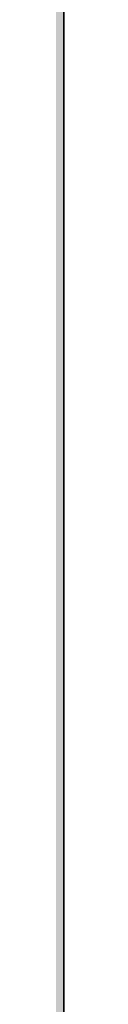
# Model space of a CAD drawing. Units: inches. Extents: x 2083 to 3317, y 1141 to 2115.
# Tile 205 of 256: x 3126.9598 to 3126.9598, y 1263.6134 to 1264.1307. Entities that reach past the tile are written whole.
import ezdxf

# ---------------------------------------------------------------- set-up
doc = ezdxf.new("R2010")
doc.units = ezdxf.units.IN
doc.layers.add('A-ANNO-DIMS', color=2, linetype='Continuous', lineweight=18)
doc.layers.add('A-WALL', color=7, linetype='Continuous', lineweight=35)
doc.layers.add('A-WALL-PATT', color=251, linetype='Continuous', lineweight=13, true_color=0x636466)
doc.styles.get("Standard").update_dxf_attribs({"font": 'arial.ttf'})
doc.dimstyles.new('ISO-25', dxfattribs={"dimtxt": 12, "dimasz": 12, "dimexe": 1.25, "dimexo": 0.625, "dimtad": 1, "dimlunit": 3, "dimtxsty": 'Standard', "dimcen": 2.5, "dimadec": 0, "dimazin": 0, "dimtfac": 1, "dimtmove": 0, "dimatfit": 3, "dimfxl": 1, "dimarcsym": 0})

# ---------------------------------------------------------------- blocks, each defined once
blk = doc.blocks.new('*D9')
at = {"layer": 'A-ANNO-DIMS', "color": 0, "lineweight": -2, "transparency": 16777216}
for p, q in [((3127.58478, 1486.76136), (3190.40309, 1486.76136)), ((3189.15309, 1474.76136), (3189.15309, 1275.26136)), ((3127.58478, 1263.26136), (3190.40309, 1263.26136))]:
    blk.add_line(p, q, dxfattribs=at)
at = {"layer": 'A-ANNO-DIMS', "color": 0, "transparency": 16777216}
for points in [[(3187.15309, 1474.76136), (3191.15309, 1474.76136), (3189.15309, 1486.76136)], [(3187.15309, 1275.26136), (3191.15309, 1275.26136), (3189.15309, 1263.26136)]]:
    blk.add_solid(points, dxfattribs=at)
at = {"layer": 'Defpoints', "color": 0, "transparency": 16777216}
for p in [(3126.95978, 1486.76136), (3126.95978, 1263.26136), (3189.15309, 1263.26136)]:
    blk.add_point(p, dxfattribs=at)
at = {"layer": 'A-ANNO-DIMS', "color": 0, "transparency": 16777216, "insert": (3182.40121, 1375.01136), "char_height": 12, "attachment_point": 5, "rotation": 90}
blk.add_mtext('18\'-7.5"', dxfattribs=at)
blk = doc.blocks.new('*D26')
at = {"layer": 'A-ANNO-DIMS', "color": 0, "lineweight": -2, "transparency": 16777216}
for p, q in [((3088.98584, 1274.91509), (3088.98584, 1270.95196)), ((3111.24004, 1274.91509), (3111.24004, 1270.95196)), ((3076.98584, 1272.20196), (2840.26245, 1272.20196)), ((3111.24004, 1272.20196), (3088.98584, 1272.20196)), ((3123.24004, 1272.20196), (3135.24004, 1272.20196))]:
    blk.add_line(p, q, dxfattribs=at)
at = {"layer": 'A-ANNO-DIMS', "color": 0, "transparency": 16777216}
for points in [[(3076.98584, 1274.20196), (3076.98584, 1270.20196), (3088.98584, 1272.20196)], [(3123.24004, 1274.20196), (3123.24004, 1270.20196), (3111.24004, 1272.20196)]]:
    blk.add_solid(points, dxfattribs=at)
at = {"layer": 'Defpoints', "color": 0, "transparency": 16777216}
for p in [(3088.98584, 1275.54009), (3111.24004, 1275.54009), (3088.98584, 1272.20196)]:
    blk.add_point(p, dxfattribs=at)
at = {"layer": 'A-ANNO-DIMS', "color": 0, "transparency": 16777216, "insert": (2952.62415, 1279.0316), "char_height": 12, "attachment_point": 5}
blk.add_mtext('NIGHTSTAND 1\'-10 1/2" TYP.', dxfattribs=at)
blk = doc.blocks.new('*D27')
at = {"layer": 'A-ANNO-DIMS', "color": 0, "lineweight": -2, "transparency": 16777216}
for p, q in [((3114.57817, 1309.79428), (3114.57817, 1321.79428)), ((3111.86504, 1297.79428), (3115.82817, 1297.79428)), ((3114.57817, 1297.79428), (3114.57817, 1275.54009)), ((3111.86504, 1275.54009), (3115.82817, 1275.54009)), ((3114.57817, 1263.54009), (3114.57817, 1140.98859))]:
    blk.add_line(p, q, dxfattribs=at)
at = {"layer": 'A-ANNO-DIMS', "color": 0, "transparency": 16777216}
for points in [[(3112.57817, 1309.79428), (3116.57817, 1309.79428), (3114.57817, 1297.79428)], [(3112.57817, 1263.54009), (3116.57817, 1263.54009), (3114.57817, 1275.54009)]]:
    blk.add_solid(points, dxfattribs=at)
at = {"layer": 'Defpoints', "color": 0, "transparency": 16777216}
for p in [(3111.24004, 1297.79428), (3111.24004, 1275.54009), (3114.57817, 1275.54009)]:
    blk.add_point(p, dxfattribs=at)
at = {"layer": 'A-ANNO-DIMS', "color": 0, "transparency": 16777216, "insert": (3107.74853, 1196.26434), "char_height": 12, "attachment_point": 5, "rotation": 90}
blk.add_mtext('1\'-10 1/2" TYP.', dxfattribs=at)

msp = doc.modelspace()

# ---------------------------------------------------------------- hatches: boundary and pattern name
at = {"layer": 'A-WALL-PATT'}
h = msp.add_hatch(color=256, dxfattribs=at)
h.dxf.hatch_style = 1
h.paths.add_polyline_path([(3126.95978, 2020.76136), (2748.95978, 2020.76136), (2604.95978, 2020.76136), (2226.95978, 2020.76136), (2226.95978, 1702.76136), (2466.95978, 1702.76136), (2466.95978, 1582.76136), (2418.95978, 1582.76136), (2418.95978, 1477.76136), (2226.95978, 1477.76136), (2226.95978, 1263.26136), (2544.95978, 1263.26136), (2544.95978, 1411.76136), (2604.95978, 1411.76136), (2685.95978, 1411.76136), (2685.95978, 1420.76136), (2604.95978, 1420.76136), (2604.95978, 1573.76136), (2604.95978, 1702.76136), (2604.95978, 2011.76136), (2748.95978, 2011.76136), (2748.95978, 1702.76136), (2862.95978, 1702.76136), (2862.95978, 1621.76136), (2871.95978, 1621.76136), (2871.95978, 1702.76136), (2883.95978, 1702.76136), (2883.95978, 1706.93946, -0.026459), (2883.95978, 1711.76136), (2757.95978, 1711.76136), (2757.95978, 1807.76136), (2787.95978, 1807.76136), (2787.95978, 1812.26136), (2757.95978, 1812.26136), (2757.95978, 2011.76136), (2877.95978, 2011.76136), (2877.95978, 1812.26136), (2847.95978, 1812.26136), (2847.95978, 1807.76136), (2889.83574, 1807.76136), (2889.83574, 1812.26136), (2882.45978, 1812.26136), (2882.45978, 2011.76136), (3117.95978, 2011.76136), (3117.95978, 1812.26136), (2937.83574, 1812.26136), (2937.83574, 1807.76136), (2995.70978, 1807.76136), (2995.70978, 1796.11767), (3000.20978, 1796.11767), (3000.20978, 1807.76136), (3117.95978, 1807.76136), (3117.95978, 1711.76136), (3000.20978, 1711.76136), (3000.20978, 1760.11767), (2998.5727, 1760.11767, -0.020711), (2995.70978, 1760.11767), (2995.70978, 1711.76136), (2931.95978, 1711.76136), (2931.95978, 1702.76136), (3126.95978, 1702.76136)])
h.paths.add_polyline_path([(2471.45978, 2011.76136), (2471.45978, 1810.01136), (2462.71694, 1810.01136), (2462.71694, 1805.51136), (2505.95978, 1805.51136), (2505.95978, 1810.01136), (2475.95978, 1810.01136), (2475.95978, 2011.76136), (2595.95978, 2011.76136), (2595.95978, 1810.01136), (2565.95978, 1810.01136), (2565.95978, 1805.51136), (2595.95978, 1805.51136), (2595.95978, 1711.76136), (2235.95978, 1711.76136), (2235.95978, 1805.51136), (2353.70978, 1805.51136), (2353.70978, 1796.05416), (2358.20978, 1796.05416), (2358.20978, 1805.51136), (2414.71694, 1805.51136), (2414.71694, 1810.01136), (2235.95978, 1810.01136), (2235.95978, 2011.76136)], flags=16)
h.paths.add_polyline_path([(2270.20473, 1994.61001), (2270.20473, 1970.61001), (2246.20473, 1970.61001), (2246.20473, 1994.61001)], flags=0)
edge = h.paths.add_edge_path(flags=0)
edge.add_ellipse((2332.02739, 1899.79818), major_axis=(-3.04299, 3.04299), ratio=0.1682525, start_angle=-161.33217, end_angle=-156.30711, ccw=False)
edge.add_ellipse((2333.08204, 1898.74353), major_axis=(-1.05465, 1.05465), ratio=0.4535321, start_angle=-123.37102, end_angle=-94.15911)
edge = h.paths.add_edge_path(flags=0)
edge.add_ellipse((2332.02739, 1968.87629), major_axis=(3.04299, 3.04299), ratio=0.1682525, start_angle=18.66783, end_angle=23.69289)
edge.add_spline(control_points=[(2332.9256, 1970.6911), (2332.22677, 1970.3361), (2330.89371, 1969.65891), (2328.41308, 1970.93214), (2327.20393, 1967.74871), (2324.7096, 1969.95559), (2322.53282, 1967.01235), (2320.01285, 1971.29581), (2317.68031, 1968.15784), (2316.04053, 1967.10205), (2315.4269, 1966.8096)], knot_values=[0, 0, 0, 0, 2.267059, 4.324559, 6.685584, 8.878641, 11.121502, 14.300359, 17.755284, 19.732645, 19.732645, 19.732645, 19.732645], degree=3, periodic=0)
edge.add_ellipse((2332.02739, 1968.87629), major_axis=(3.04299, 3.04299), ratio=0.1682525, start_angle=18.66783, end_angle=23.69289, ccw=False)
edge.add_ellipse((2333.08204, 1969.93094), major_axis=(1.05465, 1.05465), ratio=0.4535321, start_angle=56.62898, end_angle=85.84089, ccw=False)
edge = h.paths.add_edge_path(flags=0)
edge.add_spline(control_points=[(2296.42829, 1967.98791), (2293.6278, 1965.33631), (2287.70362, 1959.72709), (2299.74386, 1949.9957), (2294.53259, 1935.66853), (2290.57323, 1920.60351), (2293.39412, 1909.97369), (2296.18541, 1904.96654)], knot_values=[0.099185, 0.099185, 0.099185, 0.099185, 0.345301, 0.619822, 0.982653, 1.386093, 1.810555, 1.810555, 1.810555, 1.810555], degree=3, periodic=0)
edge.add_spline(control_points=[(2296.18541, 1904.96654), (2297.38358, 1902.6193), (2298.00097, 1901.94931), (2298.55297, 1901.46815)], knot_values=[0.006246, 0.006246, 0.006246, 0.006246, 0.055476, 0.055476, 0.055476, 0.055476], degree=3, periodic=0)
edge.add_spline(control_points=[(2298.55297, 1901.46815), (2297.25861, 1900.92322), (2295.22529, 1900.23213), (2293.06023, 1900.61421), (2292.10142, 1900.78841), (2292.08958, 1900.79057)], knot_values=[0.312835, 0.312835, 0.312835, 0.312835, 0.40178, 0.474987, 0.475903, 0.475903, 0.475903, 0.475903], degree=3, periodic=0)
edge.add_arc((2292.79365, 1904.66411), 3.93701, 215.4209, 259.69818, ccw=False)
edge.add_spline(control_points=[(2289.58531, 1902.3823), (2289.47665, 1902.53509), (2289.36848, 1902.68804), (2289.26086, 1902.84117)], knot_values=[0.102872, 0.102872, 0.102872, 0.102872, 0.116896, 0.116896, 0.116896, 0.116896], degree=3, periodic=0)
edge.add_spline(control_points=[(2289.26086, 1902.84117), (2288.6866, 1902.55019), (2287.64005, 1902.0199), (2285.88134, 1901.87395), (2283.85297, 1901.50435), (2281.71999, 1899.71054), (2278.46699, 1899.49294), (2276.15714, 1901.8832), (2272.25895, 1899.80407), (2267.77761, 1901.84318), (2262.24388, 1900.18403), (2257.41493, 1901.78206), (2254.31837, 1900.72612), (2253.17828, 1900.33734)], knot_values=[0, 0, 0, 0, 1.907977, 3.477176, 5.261074, 7.972851, 11.680248, 13.717921, 16.939592, 22.789562, 27.502503, 33.595215, 37.145618, 37.145618, 37.145618, 37.145618], degree=3, periodic=0)
edge.add_line((2253.17828, 1900.33734), (2250.24424, 1902.84117))
edge.add_line((2250.24424, 1902.84117), (2250.24424, 1965.8333))
edge.add_line((2250.24424, 1965.8333), (2253.17828, 1968.33712))
edge.add_spline(control_points=[(2253.17828, 1968.33712), (2254.31837, 1967.94835), (2257.41493, 1966.89241), (2262.24388, 1968.49043), (2267.77761, 1966.83128), (2271.52673, 1968.53722), (2273.87591, 1967.82829), (2274.2067, 1967.72764)], knot_values=[0, 0, 0, 0, 0.09018, 0.244935, 0.364644, 0.513233, 0.537855, 0.537855, 0.537855, 0.537855], degree=3, periodic=0)
edge.add_arc((2274.35289, 1963.79335), 3.93701, 72.05113, 92.12795, ccw=False)
edge.add_arc((2281.29693, 1985.23), 18.5963, 252.051134, 288.565722)
edge.add_arc((2292.31672, 1956.02888), 12.64608, 71.026788, 113.778218, ccw=False)
edge = h.paths.add_edge_path(flags=0)
edge.add_spline(control_points=[(2274.89941, 1951.85619), (2275.06616, 1951.61659), (2275.23269, 1951.37659), (2275.39799, 1951.13585)], knot_values=[1.409916, 1.409916, 1.409916, 1.409916, 1.43159, 1.43159, 1.43159, 1.43159], degree=3, periodic=0)
edge.add_spline(control_points=[(2275.39799, 1951.13585), (2275.79211, 1950.56189), (2276.17923, 1949.98377), (2276.54555, 1949.3971)], knot_values=[1.358238, 1.358238, 1.358238, 1.358238, 1.409916, 1.409916, 1.409916, 1.409916], degree=3, periodic=0)
edge.add_line((2276.54555, 1949.3971), (2277.43729, 1947.86218))
edge.add_spline(control_points=[(2277.43729, 1947.86218), (2276.30383, 1945.67311), (2274.6397, 1942.42688), (2274.63161, 1938.0939), (2272.79912, 1930.85155), (2274.35643, 1943.89705), (2275.94768, 1947.92336), (2276.54555, 1949.3971)], knot_values=[0.005632, 0.005632, 0.005632, 0.005632, 0.186014, 0.266002, 0.357087, 0.59639, 0.739732, 0.739732, 0.739732, 0.739732], degree=3, periodic=0)
edge.add_spline(control_points=[(2276.54555, 1949.3971), (2276.17923, 1949.98377), (2275.79211, 1950.56189), (2275.39799, 1951.13585)], knot_values=[1.358238, 1.358238, 1.358238, 1.358238, 1.409916, 1.409916, 1.409916, 1.409916], degree=3, periodic=0)
edge.add_spline(control_points=[(2275.39799, 1951.13585), (2274.9425, 1950.08045), (2274.20776, 1948.02527), (2273.9346, 1944.85148), (2272.46853, 1937.62749), (2273.46622, 1945.69647), (2274.70062, 1951.05947), (2274.89941, 1951.85619)], knot_values=[0.104364, 0.104364, 0.104364, 0.104364, 0.189636, 0.269624, 0.36071, 0.600013, 0.644622, 0.644622, 0.644622, 0.644622], degree=3, periodic=0)
h.paths.add_polyline_path([(2269.16751, 1963.12757, -0.357527), (2268.17063, 1960.97637, -0.092561), (2268.17063, 1939.43632, -0.357527), (2269.16751, 1937.28512, -0.357527), (2267.01631, 1938.282, -0.164785), (2254.68558, 1938.282, -0.357527), (2252.53438, 1937.28512, -0.357527), (2253.53126, 1939.43632, -0.092561), (2253.53126, 1960.97637, -0.357527), (2252.53438, 1963.12757, -0.357527), (2254.68558, 1962.13069, -0.164785), (2267.01631, 1962.13069, -0.357527)], flags=0)
h.paths.add_polyline_path([(2248.87407, 1967.8018), (2248.87407, 1957.02771), (2249.45778, 1957.02771), (2249.45778, 1911.64676), (2248.87407, 1911.64676), (2248.87407, 1900.87267), (2246.51186, 1900.87267, 0.197327), (2244.14966, 1902.45687), (2244.14966, 1966.21759, 0.197327), (2246.51186, 1967.8018)], flags=0)
h.paths.add_polyline_path([(2269.16751, 1931.38934, -0.357527), (2268.17063, 1929.23814, -0.092561), (2268.17063, 1907.6981, -0.357527), (2269.16751, 1905.54689, -0.357527), (2267.01631, 1906.54377, -0.164785), (2254.68558, 1906.54377, -0.357527), (2252.53438, 1905.54689, -0.357527), (2253.53126, 1907.6981, -0.092561), (2253.53126, 1929.23814, -0.357527), (2252.53438, 1931.38934, -0.357527), (2254.68558, 1930.39246, -0.164785), (2267.01631, 1930.39246, -0.357527)], flags=0)
edge = h.paths.add_edge_path(flags=0)
edge.add_spline(control_points=[(2276.19686, 1906.7237), (2276.16814, 1909.02893), (2276.11405, 1913.37185), (2270.59842, 1924.92498), (2273.90517, 1919.01278), (2275.92171, 1916.26206), (2275.47457, 1912.40215), (2277.25787, 1910.38062), (2276.69604, 1908.22504), (2276.64622, 1906.81302), (2276.61782, 1906.00841)], knot_values=[0, 0, 0, 0, 8.61026, 16.221274, 18.843057, 23.804898, 27.440828, 29.356102, 31.203478, 33.650687, 33.650687, 33.650687, 33.650687], degree=3, periodic=0)
edge.add_spline(control_points=[(2276.61782, 1906.00841), (2276.62331, 1905.62414), (2276.49774, 1904.62866), (2275.44178, 1903.85473), (2274.93731, 1903.08045), (2274.85908, 1902.84117)], knot_values=[0.156488, 0.156488, 0.156488, 0.156488, 0.184398, 0.231376, 0.250598, 0.250598, 0.250598, 0.250598], degree=3, periodic=0)
edge.add_line((2274.85908, 1902.84117), (2276.50598, 1902.84117))
edge.add_spline(control_points=[(2276.50598, 1902.84117), (2276.78831, 1903.08494), (2277.66507, 1904.1252), (2278.24954, 1904.34074), (2277.65387, 1908.52739), (2278.15567, 1906.22781), (2278.10046, 1905.28595), (2278.84667, 1904.06901), (2277.85679, 1903.41495), (2277.87419, 1902.99105), (2277.90356, 1902.84117)], knot_values=[0.059574, 0.059574, 0.059574, 0.059574, 0.080753, 0.103741, 0.16972, 0.176036, 0.207137, 0.240474, 0.262341, 0.27366, 0.27366, 0.27366, 0.27366], degree=3, periodic=0)
edge.add_line((2277.90356, 1902.84117), (2280.02983, 1902.84117))
edge.add_spline(control_points=[(2280.02983, 1902.84117), (2279.88822, 1903.0884), (2279.49926, 1903.98155), (2280.15228, 1905.93935), (2278.10362, 1909.65776), (2279.76239, 1907.18529), (2280.3279, 1904.87486), (2280.48511, 1903.48959), (2281.46327, 1903.24943), (2281.75834, 1902.9365), (2281.83404, 1902.84117)], knot_values=[0.013856, 0.013856, 0.013856, 0.013856, 0.034874, 0.088867, 0.107879, 0.126738, 0.158714, 0.193757, 0.217487, 0.226722, 0.226722, 0.226722, 0.226722], degree=3, periodic=0)
edge.add_spline(control_points=[(2281.83404, 1902.84117), (2281.78753, 1902.8267), (2281.64702, 1902.78299), (2281.39553, 1902.85949), (2281.08808, 1902.98524), (2280.72068, 1903.0609), (2280.33345, 1903.02573), (2280.12477, 1902.89888), (2280.02983, 1902.84117)], knot_values=[0, 0, 0, 0, 0.14413, 0.435517, 0.749276, 1.153046, 1.548371, 1.878348, 1.878348, 1.878348, 1.878348], degree=3, periodic=0)
edge.add_line((2280.02983, 1902.84117), (2277.90356, 1902.84117))
edge.add_spline(control_points=[(2277.90356, 1902.84117), (2277.89286, 1902.79586), (2277.8654, 1902.67964), (2277.60748, 1902.68748), (2277.27405, 1902.8007), (2276.83792, 1902.61977), (2276.58381, 1902.78926), (2276.50598, 1902.84117)], knot_values=[0, 0, 0, 0, 0.127189, 0.326199, 0.628009, 1.24357, 1.515331, 1.515331, 1.515331, 1.515331], degree=3, periodic=0)
edge.add_line((2276.50598, 1902.84117), (2274.85908, 1902.84117))
edge.add_spline(control_points=[(2274.85908, 1902.84117), (2274.81444, 1902.89859), (2274.72513, 1903.01345), (2274.49348, 1903.11897), (2274.24429, 1902.96054), (2273.93712, 1903.18494), (2273.61404, 1902.98314), (2273.40832, 1902.88304), (2273.32225, 1902.84117)], knot_values=[0, 0, 0, 0, 0.21843, 0.436957, 0.687977, 0.990379, 1.398396, 1.69185, 1.69185, 1.69185, 1.69185], degree=3, periodic=0)
edge.add_spline(control_points=[(2273.32225, 1902.84117), (2273.61674, 1903.44569), (2274.274, 1904.53825), (2276.02724, 1904.5737), (2276.20696, 1906.58364), (2276.19686, 1906.7237)], knot_values=[0.012227, 0.012227, 0.012227, 0.012227, 0.059472, 0.106218, 0.134458, 0.134458, 0.134458, 0.134458], degree=3, periodic=0)
h.paths.add_polyline_path([(2270.77605, 1897.78983), (2270.77605, 1873.78983), (2246.77605, 1873.78983), (2246.77605, 1897.78983)], flags=0)
h.paths.add_polyline_path([(2353.70978, 1760.00506), (2353.70978, 1760.05416), (2358.20978, 1760.05416, -0.033729)], flags=0)
h.paths.add_polyline_path([(2321.81912, 1737.52919), (2341.99533, 1737.52919, -0.414214), (2343.20327, 1736.32124), (2343.20327, 1721.0206, -0.414214), (2341.99533, 1719.81265), (2321.81912, 1719.81265, -0.414214), (2320.61117, 1721.0206), (2320.61117, 1736.32124, -0.414214)], flags=0)
h.paths.add_polyline_path([(2324.23501, 1736.32124), (2339.57944, 1736.32124, -0.414214), (2341.99533, 1733.90535), (2341.99533, 1725.44973, -0.414214), (2339.57944, 1723.03384), (2333.68059, 1723.03384), (2333.84532, 1722.04547, -0.870646), (2335.4254, 1721.82589, -0.767327), (2333.92269, 1721.42324), (2331.29102, 1721.42324, -0.767327), (2329.78832, 1721.82589, -0.870646), (2331.3684, 1722.04547), (2331.53313, 1723.03384), (2324.23501, 1723.03384, -0.414214), (2321.81912, 1725.44973), (2321.81912, 1733.90535, -0.414214)], flags=0)
h.paths.add_polyline_path([(2570.48379, 1928.61544), (2589.68379, 1928.61544), (2590.16883, 1928.61544), (2590.16883, 1904.9934), (2570.48379, 1904.9934)], flags=0)
h.paths.add_polyline_path([(2574.44732, 1927.26382, -1), (2572.82884, 1927.26382, -1)], flags=0)
h.paths.add_polyline_path([(2573.08987, 1926.94088), (2573.92503, 1927.77604), (2574.14774, 1927.55333), (2573.31258, 1926.71817)], flags=0)
h.paths.add_polyline_path([(2578.77906, 1919.72962, -1), (2571.59166, 1919.72962, -1)], flags=0)
h.paths.add_polyline_path([(2578.38536, 1919.72962, -1), (2571.98536, 1919.72962, -1)], flags=0)
h.paths.add_polyline_path([(2331.59576, 1729.47622, -1), (2333.61795, 1729.47622, -1)], flags=0)
h.paths.add_polyline_path([(2578.03423, 1927.26382, -1), (2576.41574, 1927.26382, -1)], flags=0)
h.paths.add_polyline_path([(2576.68885, 1927.53109), (2576.91156, 1927.7538), (2577.74673, 1926.91863), (2577.52402, 1926.69592)], flags=0)
h.paths.add_polyline_path([(2578.13906, 1909.85954, -1), (2572.23166, 1909.85954, -1)], flags=0)
h.paths.add_polyline_path([(2577.74536, 1909.85954, -1), (2572.62536, 1909.85954, -1)], flags=0)
h.paths.add_polyline_path([(2583.79772, 1927.26382, -1), (2582.17923, 1927.26382, -1)], flags=0)
h.paths.add_polyline_path([(2582.71865, 1927.7538), (2583.55381, 1926.91863), (2583.3311, 1926.69592), (2582.49594, 1927.53109)], flags=0)
h.paths.add_polyline_path([(2582.49594, 1927.53109), (2582.71865, 1927.7538), (2583.55381, 1926.91863), (2583.3311, 1926.69592)], flags=0)
h.paths.add_polyline_path([(2587.73906, 1920.52962, -1), (2581.83166, 1920.52962, -1)], flags=0)
h.paths.add_polyline_path([(2587.34536, 1920.52962, -1), (2582.22536, 1920.52962, -1)], flags=0)
h.paths.add_polyline_path([(2587.38462, 1927.26382, -1), (2585.76613, 1927.26382, -1)], flags=0)
h.paths.add_polyline_path([(2586.08199, 1926.98025), (2586.91716, 1927.81541), (2587.13987, 1927.5927), (2586.3047, 1926.75754)], flags=0)
h.paths.add_polyline_path([(2588.37906, 1910.65954, -1), (2581.19166, 1910.65954, -1)], flags=0)
h.paths.add_polyline_path([(2587.98536, 1910.65954, -1), (2581.58536, 1910.65954, -1)], flags=0)
h.paths.add_polyline_path([(2417.16773, 1729.4779), (2437.34394, 1729.4779, -0.414214), (2438.55188, 1728.26995), (2438.55188, 1712.96931, -0.414214), (2437.34394, 1711.76136), (2417.16773, 1711.76136, -0.414214), (2415.95978, 1712.96931), (2415.95978, 1728.26995, -0.414214)], flags=0)
h.paths.add_polyline_path([(2419.58362, 1728.26995), (2434.92805, 1728.26995, -0.414214), (2437.34394, 1725.85406), (2437.34394, 1717.39844, -0.414214), (2434.92805, 1714.98255), (2429.0292, 1714.98255), (2429.19393, 1713.99418, -0.870646), (2430.77401, 1713.7746, -0.767327), (2429.2713, 1713.37195), (2426.63963, 1713.37195, -0.767327), (2425.13693, 1713.7746, -0.870646), (2426.71701, 1713.99418), (2426.88174, 1714.98255), (2419.58362, 1714.98255, -0.414214), (2417.16773, 1717.39844), (2417.16773, 1725.85406, -0.414214)], flags=0)
h.paths.add_polyline_path([(2419.58362, 1728.26995), (2434.92805, 1728.26995, -0.414214), (2437.34394, 1725.85406), (2437.34394, 1717.39844, -0.414214), (2434.92805, 1714.98255), (2429.0292, 1714.98255), (2428.35812, 1719.00903), (2427.55282, 1719.00903), (2426.88174, 1714.98255), (2419.58362, 1714.98255, -0.414214), (2417.16773, 1717.39844), (2417.16773, 1725.85406, -0.414214)], flags=0)
h.paths.add_polyline_path([(2426.94437, 1721.42492, -1), (2428.96656, 1721.42492, -1)], flags=0)
h.paths.add_polyline_path([(2475.95978, 1702.76136), (2595.95978, 1702.76136), (2595.95978, 1582.76136), (2475.95978, 1582.76136)], flags=16)
h.paths.add_polyline_path([(2427.95978, 1573.76136), (2595.95978, 1573.76136), (2595.95978, 1468.76136), (2595.95978, 1420.76136), (2384.45978, 1420.76136), (2384.45978, 1468.76136), (2427.95978, 1468.76136)], flags=16)
h.paths.add_polyline_path([(2379.95978, 1468.76136), (2379.95978, 1420.76136), (2235.95978, 1420.76136), (2235.95978, 1468.76136)], flags=16)
h.paths.add_polyline_path([(2317.816, 1466.69577), (2337.9922, 1466.69577, -0.414214), (2339.20015, 1465.48782), (2339.20015, 1450.18718, -0.414214), (2337.9922, 1448.97923), (2317.816, 1448.97923, -0.414214), (2316.60805, 1450.18718), (2316.60805, 1465.48782, -0.414214)], flags=0)
h.paths.add_polyline_path([(2320.23189, 1465.48782), (2335.57631, 1465.48782, -0.414214), (2337.9922, 1463.07193), (2337.9922, 1454.61631, -0.414214), (2335.57631, 1452.20042), (2329.67747, 1452.20042), (2329.84219, 1451.21205, -0.870646), (2331.42228, 1450.99247, -0.767327), (2329.91957, 1450.58983), (2327.2879, 1450.58983, -0.767327), (2325.7852, 1450.99247, -0.870646), (2327.36528, 1451.21205), (2327.53001, 1452.20042), (2320.23189, 1452.20042, -0.414214), (2317.816, 1454.61631), (2317.816, 1463.07193, -0.414214)], flags=0)
h.paths.add_polyline_path([(2320.23189, 1465.48782), (2335.57631, 1465.48782, -0.414214), (2337.9922, 1463.07193), (2337.9922, 1454.61631, -0.414214), (2335.57631, 1452.20042), (2329.67747, 1452.20042), (2329.00638, 1456.22691), (2328.20109, 1456.22691), (2327.53001, 1452.20042), (2320.23189, 1452.20042, -0.414214), (2317.816, 1454.61631), (2317.816, 1463.07193, -0.414214)], flags=0)
h.paths.add_polyline_path([(2327.59264, 1458.6428, -1), (2329.61483, 1458.6428, -1)], flags=0)
h.paths.add_polyline_path([(2244.41174, 1433.34045), (2241.92094, 1433.34045, -0.414214), (2240.01786, 1435.24354), (2240.01786, 1440.95281, -0.414211), (2241.92093, 1442.8559), (2244.41174, 1442.8559, -1.976472)], flags=0)
h.paths.add_polyline_path([(2245.35689, 1434.39754, -0.414214), (2245.35689, 1441.79881, -2.144098)], flags=0)
h.paths.add_polyline_path([(2535.95978, 1416.26136), (2535.95978, 1272.26136), (2235.95978, 1272.26136), (2235.95978, 1416.26136)], flags=16)
h.paths.add_polyline_path([(2260.11956, 1384.29284), (2260.11956, 1362.03865), (2237.86537, 1362.03865), (2237.86537, 1384.29284)], flags=0)
edge = h.paths.add_edge_path(flags=0)
edge.add_line((2318.25185, 1362.0933), (2318.1458, 1362.00097))
edge.add_ellipse((2317.44512, 1360.43104), major_axis=(2.82164, 2.82164), ratio=0.1682525, start_angle=18.66783, end_angle=20.94813, ccw=False)
edge.add_ellipse((2318.42305, 1361.40897), major_axis=(0.97793, 0.97793), ratio=0.4535321, start_angle=56.62898, end_angle=70.2262, ccw=False)
edge = h.paths.add_edge_path(flags=0)
edge.add_line((2319.10737, 1295.57108), (2319.01504, 1295.67713))
edge.add_ellipse((2317.44512, 1296.37781), major_axis=(-2.82164, 2.82164), ratio=0.1682525, start_angle=-161.33217, end_angle=-159.05187, ccw=False)
edge.add_ellipse((2318.42305, 1295.39988), major_axis=(-0.97793, 0.97793), ratio=0.4535321, start_angle=-123.37102, end_angle=-109.7738)
edge = h.paths.add_edge_path(flags=0)
edge.add_spline(control_points=[(2284.21035, 1301.17022), (2284.58069, 1300.44472), (2284.89119, 1299.89202), (2285.15955, 1299.46102)], knot_values=[0.039066, 0.039066, 0.039066, 0.039066, 0.055476, 0.055476, 0.055476, 0.055476], degree=3, periodic=0)
edge.add_line((2285.15955, 1299.46102), (2284.21035, 1301.17022))
edge = h.paths.add_edge_path(flags=0)
edge.add_line((2280.41246, 1297.29801), (2283.36999, 1297.03612))
edge.add_line((2283.36999, 1297.03612), (2286.40569, 1297.92631))
edge.add_spline(control_points=[(2286.40569, 1297.92631), (2285.30549, 1297.46312), (2284.34478, 1297.12915), (2283.36999, 1297.03612)], knot_values=[0.394369, 0.394369, 0.394369, 0.394369, 0.475903, 0.475903, 0.475903, 0.475903], degree=3, periodic=0)
edge.add_spline(control_points=[(2283.36999, 1297.03612), (2283.28139, 1297.02767), (2282.31629, 1296.95734), (2281.3125, 1297.13448), (2280.42344, 1297.29602), (2280.41246, 1297.29801)], knot_values=[0.312835, 0.312835, 0.312835, 0.312835, 0.320246, 0.393453, 0.394369, 0.394369, 0.394369, 0.394369], degree=3, periodic=0)
edge = h.paths.add_edge_path(flags=0)
edge.add_line((2284.43556, 1359.60729), (2280.44629, 1355.32805))
edge.add_line((2280.44629, 1355.32805), (2279.57999, 1351.01775))
edge.add_line((2279.57999, 1351.01775), (2282.41297, 1346.58043))
edge.add_spline(control_points=[(2282.41297, 1346.58043), (2283.15333, 1345.58924), (2284.2529, 1344.0289), (2284.80104, 1342.38717), (2284.93516, 1341.80554)], knot_values=[1.240098, 1.240098, 1.240098, 1.240098, 1.332892, 1.382712, 1.382712, 1.382712, 1.382712], degree=3, periodic=0)
edge.add_spline(control_points=[(2284.93516, 1341.80554), (2285.31911, 1340.1406), (2285.23303, 1338.4092), (2284.90994, 1336.65412)], knot_values=[1.097484, 1.097484, 1.097484, 1.097484, 1.240098, 1.240098, 1.240098, 1.240098], degree=3, periodic=0)
edge.add_spline(control_points=[(2284.90994, 1336.65412), (2284.58685, 1334.89904), (2284.02675, 1333.12027), (2283.46264, 1331.36058)], knot_values=[0.95487, 0.95487, 0.95487, 0.95487, 1.097484, 1.097484, 1.097484, 1.097484], degree=3, periodic=0)
edge.add_line((2283.46264, 1331.36058), (2281.89038, 1326.15336))
edge.add_line((2281.89038, 1326.15336), (2280.75626, 1321.05609))
edge.add_line((2280.75626, 1321.05609), (2280.2992, 1316.00198))
edge.add_line((2280.2992, 1316.00198), (2280.71593, 1310.95007))
edge.add_line((2280.71593, 1310.95007), (2282.02809, 1305.97214))
edge.add_line((2282.02809, 1305.97214), (2284.21035, 1301.17022))
edge.add_spline(control_points=[(2284.21035, 1301.17022), (2283.34073, 1302.73019), (2282.6119, 1304.33649), (2282.02809, 1305.97214)], knot_values=[0.099185, 0.099185, 0.099185, 0.099185, 0.241799, 0.241799, 0.241799, 0.241799], degree=3, periodic=0)
edge.add_spline(control_points=[(2282.02809, 1305.97214), (2281.44428, 1307.60778), (2281.00549, 1309.27276), (2280.71593, 1310.95007)], knot_values=[0.241799, 0.241799, 0.241799, 0.241799, 0.384413, 0.384413, 0.384413, 0.384413], degree=3, periodic=0)
edge.add_spline(control_points=[(2280.71593, 1310.95007), (2280.43324, 1312.58761), (2280.28939, 1314.27696), (2280.29889, 1315.96203), (2280.2992, 1316.00198)], knot_values=[0.384413, 0.384413, 0.384413, 0.384413, 0.523647, 0.527028, 0.527028, 0.527028, 0.527028], degree=3, periodic=0)
edge.add_spline(control_points=[(2280.2992, 1316.00198), (2280.31233, 1317.68696), (2280.47787, 1319.36793), (2280.75626, 1321.05609)], knot_values=[0.527028, 0.527028, 0.527028, 0.527028, 0.669642, 0.669642, 0.669642, 0.669642], degree=3, periodic=0)
edge.add_spline(control_points=[(2280.75626, 1321.05609), (2281.03465, 1322.74425), (2281.42588, 1324.43961), (2281.89038, 1326.15336)], knot_values=[0.669642, 0.669642, 0.669642, 0.669642, 0.812256, 0.812256, 0.812256, 0.812256], degree=3, periodic=0)
edge.add_spline(control_points=[(2281.89038, 1326.15336), (2282.26438, 1327.53325), (2282.78787, 1329.26181), (2283.35275, 1331.01778), (2283.46264, 1331.36058)], knot_values=[0.812256, 0.812256, 0.812256, 0.812256, 0.927087, 0.95487, 0.95487, 0.95487, 0.95487], degree=3, periodic=0)
edge.add_line((2283.46264, 1331.36058), (2284.90994, 1336.65412))
edge.add_line((2284.90994, 1336.65412), (2284.93516, 1341.80554))
edge.add_line((2284.93516, 1341.80554), (2282.41297, 1346.58043))
edge.add_spline(control_points=[(2282.41297, 1346.58043), (2281.27513, 1348.10379), (2280.07845, 1349.57032), (2279.57999, 1351.01775)], knot_values=[1.382712, 1.382712, 1.382712, 1.382712, 1.525326, 1.525326, 1.525326, 1.525326], degree=3, periodic=0)
edge.add_spline(control_points=[(2279.57999, 1351.01775), (2279.44328, 1351.41472), (2279.13631, 1352.85692), (2279.73519, 1354.29039), (2280.44629, 1355.32805)], knot_values=[1.525326, 1.525326, 1.525326, 1.525326, 1.564439, 1.667941, 1.667941, 1.667941, 1.667941], degree=3, periodic=0)
edge.add_spline(control_points=[(2280.44629, 1355.32805), (2281.42611, 1356.75784), (2282.93084, 1358.18256), (2284.43556, 1359.60729)], knot_values=[1.667941, 1.667941, 1.667941, 1.667941, 1.810555, 1.810555, 1.810555, 1.810555], degree=3, periodic=0)
edge.add_arc((2280.62307, 1348.51818), 11.72618, 71.026788, 113.778218)
edge.add_arc((2270.40489, 1375.59516), 17.24357, 252.051134, 288.565722, ccw=False)
edge.add_arc((2263.96597, 1355.71785), 3.65062, 72.05113, 92.12795)
edge.add_arc((2263.96597, 1355.71785), 3.65062, 92.12795, 177.98513)
edge.add_spline(control_points=[(2260.3176, 1355.8462), (2260.26042, 1354.22067), (2260.55128, 1350.18655), (2262.99934, 1346.76625), (2264.47274, 1344.64902)], knot_values=[1.43159, 1.43159, 1.43159, 1.43159, 1.564144, 1.770695, 1.770695, 1.770695, 1.770695], degree=3, periodic=0)
edge.add_line((2264.47274, 1344.64902), (2264.93559, 1343.98253))
edge.add_spline(control_points=[(2263.80104, 1340.24811), (2263.84324, 1340.51409), (2264.06724, 1341.75647), (2264.51269, 1343.00245), (2264.93505, 1343.98108)], knot_values=[0.53657, 0.53657, 0.53657, 0.53657, 0.559349, 0.644622, 0.644622, 0.644622, 0.644622], degree=3, periodic=0)
edge.add_spline(control_points=[(2264.93505, 1343.98108), (2265.11777, 1343.71497), (2265.29888, 1343.44791), (2265.47676, 1343.17936)], knot_values=[1.384077, 1.384077, 1.384077, 1.384077, 1.409916, 1.409916, 1.409916, 1.409916], degree=3, periodic=0)
edge.add_spline(control_points=[(2265.47676, 1343.17936), (2265.65464, 1342.91082), (2265.8293, 1342.64081), (2265.99913, 1342.36881)], knot_values=[1.358238, 1.358238, 1.358238, 1.358238, 1.384077, 1.384077, 1.384077, 1.384077], degree=3, periodic=0)
edge.add_line((2265.99913, 1342.36881), (2266.82601, 1340.94555))
edge.add_spline(control_points=[(2266.82601, 1340.94555), (2268.8944, 1337.08969), (2271.39817, 1325.843), (2270.51616, 1310.56856), (2275.91938, 1301.86061), (2277.78951, 1299.19945)], knot_values=[0.116896, 0.116896, 0.116896, 0.116896, 0.472987, 1.050969, 1.313793, 1.313793, 1.313793, 1.313793], degree=3, periodic=0)
edge.add_spline(control_points=[(2277.78951, 1299.19945), (2277.83941, 1299.12845), (2277.88943, 1299.0575), (2277.93957, 1298.98658)], knot_values=[0.109884, 0.109884, 0.109884, 0.109884, 0.116896, 0.116896, 0.116896, 0.116896], degree=3, periodic=0)
edge.add_line((2277.93957, 1298.98658), (2277.78885, 1299.19911))
edge.add_spline(control_points=[(2277.78885, 1299.19911), (2277.25658, 1298.92941), (2276.28635, 1298.4379), (2275.03935, 1298.33442), (2274.38333, 1298.2389), (2274.21525, 1298.20934)], knot_values=[33.12187, 33.12187, 33.12187, 33.12187, 35.029056, 36.598255, 37.144827, 37.144827, 37.144827, 37.144827], degree=3, periodic=0)
edge.add_line((2274.21525, 1298.20934), (2273.07315, 1297.89296))
edge.add_spline(control_points=[(2273.07315, 1297.89296), (2272.32294, 1297.57978), (2271.03915, 1296.51051), (2269.24839, 1296.22606), (2268.4231, 1296.37465)], knot_values=[26.532584, 26.532584, 26.532584, 26.532584, 29.198919, 31.839101, 31.839101, 31.839101, 31.839101], degree=3, periodic=0)
edge.add_line((2268.4231, 1296.37465), (2263.8785, 1297.45753))
edge.add_spline(control_points=[(2263.8785, 1297.45753), (2263.55608, 1297.35943), (2261.86031, 1296.83869), (2260.23878, 1297.28241), (2258.93345, 1297.51646)], knot_values=[15.919551, 15.919551, 15.919551, 15.919551, 16.939592, 21.226067, 21.226067, 21.226067, 21.226067], degree=3, periodic=0)
edge.add_line((2258.93345, 1297.51646), (2254.05523, 1297.32901))
edge.add_spline(control_points=[(2254.05523, 1297.32901), (2253.75553, 1297.29582), (2252.11368, 1297.16517), (2250.46187, 1297.54422), (2249.12969, 1297.66788)], knot_values=[5.306517, 5.306517, 5.306517, 5.306517, 6.276435, 10.613034, 10.613034, 10.613034, 10.613034], degree=3, periodic=0)
edge.add_line((2249.12969, 1297.66788), (2244.33165, 1296.87776))
edge.add_line((2244.33165, 1296.87776), (2241.61103, 1299.19945))
edge.add_line((2241.61103, 1299.19945), (2241.61103, 1357.6094))
edge.add_line((2241.61103, 1357.6094), (2244.33165, 1359.9311))
edge.add_line((2244.33165, 1359.9311), (2252.72882, 1359.54269))
edge.add_spline(control_points=[(2252.72882, 1359.54269), (2252.87094, 1359.54644), (2253.30574, 1359.54817), (2253.73984, 1359.51427), (2254.03174, 1359.48243)], knot_values=[0.233291, 0.233291, 0.233291, 0.233291, 0.244935, 0.268927, 0.268927, 0.268927, 0.268927], degree=3, periodic=0)
edge.add_line((2254.03174, 1359.48243), (2259.58719, 1359.41639))
edge.add_spline(control_points=[(2259.58719, 1359.41639), (2260.67707, 1359.6285), (2262.0732, 1359.897), (2263.52369, 1359.45928), (2263.83042, 1359.36595)], knot_values=[0.422516, 0.422516, 0.422516, 0.422516, 0.513233, 0.537855, 0.537855, 0.537855, 0.537855], degree=3, periodic=0)
edge.add_arc((2263.96597, 1355.71785), 3.65062, 72.05113, 92.12795, ccw=False)
edge.add_arc((2270.40489, 1375.59516), 17.24357, 252.051134, 288.565722)
edge.add_arc((2280.62307, 1348.51818), 11.72618, 71.026788, 113.778218, ccw=False)
h.paths.add_polyline_path([(2240.34053, 1359.43471), (2240.34053, 1349.44435), (2240.88178, 1349.44435), (2240.88178, 1307.3645), (2240.34053, 1307.3645), (2240.34053, 1297.37414), (2238.15016, 1297.37414, 0.197327), (2235.95978, 1298.84311), (2235.95978, 1357.96575, 0.197327), (2238.15016, 1359.43471)], flags=0)
h.paths.add_polyline_path([(2259.15779, 1355.1005, -0.357527), (2258.23342, 1353.10578, -0.092561), (2258.23342, 1333.1326, -0.357527), (2259.15779, 1331.13788, -0.357527), (2257.16307, 1332.06225, -0.164785), (2245.7293, 1332.06225, -0.357527), (2243.73458, 1331.13788, -0.357527), (2244.65895, 1333.1326, -0.092561), (2244.65895, 1353.10578, -0.357527), (2243.73458, 1355.1005, -0.357527), (2245.7293, 1354.17613, -0.164785), (2257.16307, 1354.17613, -0.357527)], flags=0)
edge = h.paths.add_edge_path(flags=0)
edge.add_line((2265.99913, 1342.36881), (2266.82601, 1340.94555))
edge.add_line((2266.82601, 1340.94555), (2265.30756, 1337.81407))
edge.add_line((2265.30756, 1337.81407), (2264.35823, 1334.65294))
edge.add_line((2264.35823, 1334.65294), (2264.26201, 1333.7997))
edge.add_spline(control_points=[(2264.26201, 1333.7997), (2264.20836, 1333.18705), (2264.16206, 1332.36553), (2264.00714, 1331.41393), (2263.96905, 1331.20183)], knot_values=[0.464444, 0.464444, 0.464444, 0.464444, 0.516691, 0.531608, 0.531608, 0.531608, 0.531608], degree=3, periodic=0)
edge.add_spline(control_points=[(2263.96905, 1331.20183), (2263.77453, 1330.11887), (2263.42437, 1328.79084), (2263.25742, 1328.53065), (2263.23403, 1328.51461)], knot_values=[0.372682, 0.372682, 0.372682, 0.372682, 0.44885, 0.464444, 0.464444, 0.464444, 0.464444], degree=3, periodic=0)
edge.add_spline(control_points=[(2263.23403, 1328.51461), (2263.09638, 1328.42023), (2263.13117, 1329.30148), (2263.27495, 1330.61575)], knot_values=[0.280919, 0.280919, 0.280919, 0.280919, 0.372682, 0.372682, 0.372682, 0.372682], degree=3, periodic=0)
edge.add_spline(control_points=[(2263.27495, 1330.61575), (2263.41874, 1331.93002), (2263.67152, 1333.67732), (2263.96985, 1335.31503)], knot_values=[0.189157, 0.189157, 0.189157, 0.189157, 0.280919, 0.280919, 0.280919, 0.280919], degree=3, periodic=0)
edge.add_spline(control_points=[(2263.96985, 1335.31503), (2264.1005, 1336.03219), (2264.41878, 1337.62191), (2264.75485, 1338.86443), (2264.94742, 1339.49112)], knot_values=[0.097394, 0.097394, 0.097394, 0.097394, 0.137578, 0.189157, 0.189157, 0.189157, 0.189157], degree=3, periodic=0)
edge.add_spline(control_points=[(2264.94742, 1339.49112), (2265.29002, 1340.60605), (2265.64424, 1341.494), (2265.99913, 1342.36881)], knot_values=[0.005632, 0.005632, 0.005632, 0.005632, 0.097394, 0.097394, 0.097394, 0.097394], degree=3, periodic=0)
h.paths.add_polyline_path([(2259.15779, 1325.67097, -0.357527), (2258.23342, 1323.67625, -0.092561), (2258.23342, 1303.70307, -0.357527), (2259.15779, 1301.70835, -0.357527), (2257.16307, 1302.63272, -0.164785), (2245.7293, 1302.63272, -0.357527), (2243.73458, 1301.70835, -0.357527), (2244.65895, 1303.70307, -0.092561), (2244.65895, 1323.67625, -0.357527), (2243.73458, 1325.67097, -0.357527), (2245.7293, 1324.74661, -0.164785), (2257.16307, 1324.74661, -0.357527)], flags=0)
edge = h.paths.add_edge_path(flags=0)
edge.add_spline(control_points=[(2261.70894, 1317.31142), (2261.67948, 1317.41758), (2261.76186, 1317.38853), (2262.49074, 1316.08987), (2262.96218, 1315.3009)], knot_values=[14.955861, 14.955861, 14.955861, 14.955861, 16.221274, 18.694826, 18.694826, 18.694826, 18.694826], degree=3, periodic=0)
edge.add_spline(control_points=[(2262.96218, 1315.3009), (2262.99044, 1315.25362), (2263.7021, 1314.06738), (2264.34898, 1313.12715), (2264.73005, 1312.16415)], knot_values=[18.694826, 18.694826, 18.694826, 18.694826, 18.843057, 22.433791, 22.433791, 22.433791, 22.433791], degree=3, periodic=0)
edge.add_spline(control_points=[(2264.73005, 1312.16415), (2264.87556, 1311.79644), (2265.17687, 1310.76981), (2265.14307, 1309.55926), (2265.24774, 1308.82419)], knot_values=[22.433791, 22.433791, 22.433791, 22.433791, 23.804898, 26.172756, 26.172756, 26.172756, 26.172756], degree=3, periodic=0)
edge.add_line((2265.24774, 1308.82419), (2265.85077, 1307.17189))
edge.add_spline(control_points=[(2265.85077, 1307.17189), (2266.06502, 1306.82168), (2266.38439, 1306.33225), (2266.4244, 1305.78055), (2266.42037, 1305.61122)], knot_values=[28.062562, 28.062562, 28.062562, 28.062562, 29.356102, 29.911721, 29.911721, 29.911721, 29.911721], degree=3, periodic=0)
edge.add_spline(control_points=[(2266.42037, 1305.61122), (2266.41612, 1305.43259), (2266.394, 1305.25), (2266.36478, 1305.06586)], knot_values=[29.911721, 29.911721, 29.911721, 29.911721, 30.497837, 30.497837, 30.497837, 30.497837], degree=3, periodic=0)
edge.add_line((2266.36478, 1305.06586), (2266.06615, 1302.1363))
edge.add_spline(control_points=[(2266.06615, 1302.1363), (2266.07124, 1301.77998), (2265.99808, 1301.19998), (2265.66327, 1300.75896), (2265.50891, 1300.58588)], knot_values=[0.156488, 0.156488, 0.156488, 0.156488, 0.184398, 0.203543, 0.203543, 0.203543, 0.203543], degree=3, periodic=0)
edge.add_line((2265.50891, 1300.58588), (2264.43534, 1299.19945))
edge.add_line((2264.43534, 1299.19945), (2265.96244, 1299.19945))
edge.add_line((2265.96244, 1299.19945), (2267.33599, 1301.17528))
edge.add_line((2267.33599, 1301.17528), (2267.31167, 1301.98624))
edge.add_spline(control_points=[(2267.31167, 1301.98624), (2267.26111, 1302.8624), (2267.16021, 1303.73713), (2267.27149, 1303.3259)], knot_values=[0.126229, 0.126229, 0.126229, 0.126229, 0.166617, 0.166617, 0.166617, 0.166617], degree=3, periodic=0)
edge.add_spline(control_points=[(2267.27149, 1303.3259), (2267.28003, 1303.2943), (2267.30979, 1303.17537), (2267.37345, 1302.88361), (2267.40612, 1302.68283), (2267.41793, 1302.60103)], knot_values=[0.166617, 0.166617, 0.166617, 0.166617, 0.16972, 0.176036, 0.180765, 0.180765, 0.180765, 0.180765], degree=3, periodic=0)
edge.add_spline(control_points=[(2267.74389, 1300.9875), (2267.68758, 1301.15094), (2267.48052, 1301.65666), (2267.48375, 1302.14479), (2267.41793, 1302.60103)], knot_values=[0.180765, 0.180765, 0.180765, 0.180765, 0.193767, 0.220139, 0.220139, 0.220139, 0.220139], degree=3, periodic=0)
edge.add_line((2267.41793, 1302.60103), (2267.74389, 1300.9875))
edge.add_spline(control_points=[(2267.74389, 1300.9875), (2267.83196, 1300.73188), (2267.93202, 1300.3099), (2267.55484, 1299.97452), (2267.42937, 1299.82921)], knot_values=[0.220139, 0.220139, 0.220139, 0.220139, 0.240474, 0.25489, 0.25489, 0.25489, 0.25489], degree=3, periodic=0)
edge.add_line((2267.42937, 1299.82921), (2267.25836, 1299.19945))
edge.add_line((2267.25836, 1299.19945), (2269.22996, 1299.19945))
edge.add_spline(control_points=[(2269.22996, 1299.19945), (2269.09865, 1299.42869), (2268.84277, 1300.01625), (2269.01157, 1300.91592), (2268.9468, 1301.66074)], knot_values=[0.013856, 0.013856, 0.013856, 0.013856, 0.034874, 0.067073, 0.067073, 0.067073, 0.067073], degree=3, periodic=0)
edge.add_line((2268.9468, 1301.66074), (2268.43158, 1303.60311))
edge.add_spline(control_points=[(2268.43158, 1303.60311), (2268.1756, 1304.19237), (2267.59621, 1305.2513), (2268.0407, 1304.62321), (2268.25139, 1304.28242)], knot_values=[0.090155, 0.090155, 0.090155, 0.090155, 0.107879, 0.120289, 0.120289, 0.120289, 0.120289], degree=3, periodic=0)
edge.add_spline(control_points=[(2268.25139, 1304.28242), (2268.36088, 1304.10533), (2269.05775, 1302.91798), (2269.38269, 1301.59042), (2269.52141, 1300.77593), (2269.57522, 1300.55578)], knot_values=[0.120289, 0.120289, 0.120289, 0.120289, 0.126738, 0.158714, 0.173506, 0.173506, 0.173506, 0.173506], degree=3, periodic=0)
edge.add_line((2269.57522, 1300.55578), (2270.6858, 1299.42126))
edge.add_spline(control_points=[(2270.6858, 1299.42126), (2270.76722, 1299.35725), (2270.83785, 1299.2814), (2270.90292, 1299.19945)], knot_values=[0.21816, 0.21816, 0.21816, 0.21816, 0.226722, 0.226722, 0.226722, 0.226722], degree=3, periodic=0)
edge.add_line((2270.9372, 1299.19291), (2270.90292, 1299.19945))
edge.add_spline(control_points=[(2270.90292, 1299.19945), (2270.85981, 1299.18603), (2270.72951, 1299.1455), (2270.49631, 1299.21644), (2270.27166, 1299.30832), (2270.12102, 1299.34796), (2270.06334, 1299.35956)], knot_values=[0.939174, 0.939174, 0.939174, 0.939174, 1.083304, 1.374691, 1.68845, 1.878348, 1.878348, 1.878348, 1.878348], degree=3, periodic=0)
edge.add_line((2270.06334, 1299.35956), (2269.22996, 1299.19945))
edge.add_line((2269.22996, 1299.19945), (2267.25836, 1299.19945))
edge.add_spline(control_points=[(2267.25836, 1299.19945), (2267.24843, 1299.15743), (2267.22297, 1299.04967), (2266.98382, 1299.05694), (2266.80921, 1299.11623), (2266.6769, 1299.10909), (2266.63653, 1299.10481)], knot_values=[0.757665, 0.757665, 0.757665, 0.757665, 0.884854, 1.083864, 1.385675, 1.515331, 1.515331, 1.515331, 1.515331], degree=3, periodic=0)
edge.add_spline(control_points=[(2266.63653, 1299.10481), (2266.48522, 1299.08879), (2266.23581, 1299.01712), (2266.03461, 1299.15132), (2265.96244, 1299.19945)], knot_values=[0, 0, 0, 0, 0.485905, 0.757665, 0.757665, 0.757665, 0.757665], degree=3, periodic=0)
edge.add_line((2265.96244, 1299.19945), (2264.43534, 1299.19945))
edge.add_line((2264.43534, 1299.19945), (2263.85844, 1299.36712))
edge.add_spline(control_points=[(2263.85844, 1299.36712), (2263.81894, 1299.37091), (2263.77953, 1299.38572), (2263.74013, 1299.4015)], knot_values=[0.845925, 0.845925, 0.845925, 0.845925, 0.978627, 0.978627, 0.978627, 0.978627], degree=3, periodic=0)
edge.add_line((2263.72179, 1299.39643), (2263.01031, 1299.19945))
edge.add_spline(control_points=[(2263.01031, 1299.19945), (2263.24579, 1299.68286), (2263.50603, 1300.12811), (2263.87349, 1300.40803)], knot_values=[0.012227, 0.012227, 0.012227, 0.012227, 0.052971, 0.052971, 0.052971, 0.052971], degree=3, periodic=0)
edge.add_spline(control_points=[(2263.87349, 1300.40803), (2263.93213, 1300.4527), (2264.08424, 1300.55298), (2264.25519, 1300.62422), (2264.35969, 1300.66475)], knot_values=[0.052971, 0.052971, 0.052971, 0.052971, 0.059472, 0.069086, 0.069086, 0.069086, 0.069086], degree=3, periodic=0)
edge.add_line((2264.35969, 1300.66475), (2265.1419, 1301.07777))
edge.add_line((2265.1419, 1301.07777), (2265.67581, 1302.79956))
edge.add_line((2265.67581, 1302.79956), (2265.5407, 1305.70407))
edge.add_line((2265.5407, 1305.70407), (2264.80307, 1309.32772))
edge.add_line((2264.80307, 1309.32772), (2263.04053, 1314.09179))
edge.add_spline(control_points=[(2263.04053, 1314.09179), (2262.38357, 1315.67144), (2261.79597, 1316.99775), (2261.70894, 1317.31142)], knot_values=[11.216896, 11.216896, 11.216896, 11.216896, 14.955861, 14.955861, 14.955861, 14.955861], degree=3, periodic=0)
h.paths.add_polyline_path([(2871.95978, 1416.26136), (2895.91005, 1416.26136), (2895.91005, 1420.76136), (2871.95978, 1420.76136), (2871.95978, 1501.76136), (2862.95978, 1501.76136), (2862.95978, 1420.76136), (2805.95978, 1420.76136), (2805.95978, 1411.76136), (2862.95978, 1411.76136), (2862.95978, 1263.26136), (3126.95978, 1263.26136), (3126.95978, 1411.76136), (3126.95978, 1486.76136), (2943.95978, 1486.76136), (2943.95978, 1477.76136), (2967.86031, 1477.76136), (2967.86031, 1420.76136), (2943.91005, 1420.76136), (2943.91005, 1416.26136), (3117.95978, 1416.26136), (3117.95978, 1420.76136), (2972.36031, 1420.76136), (2972.36031, 1477.76136), (3117.95978, 1477.76136), (3117.95978, 1420.76136), (3117.95978, 1272.26136), (2871.95978, 1272.26136)], flags=0)
h.paths.add_polyline_path([(2457.12563, 1485.94251), (2527.60265, 1485.94251), (2527.60265, 1537.6357), (2457.12563, 1537.6357)], flags=8)
h.paths.add_polyline_path([(2481.00506, 1609.9818), (2590.76582, 1609.9818), (2590.76582, 1682.00336), (2481.00506, 1682.00336)], flags=8)
h.paths.add_polyline_path([(2483.08502, 1729.12678), (2553.56205, 1729.12678), (2553.56205, 1780.81998), (2483.08502, 1780.81998)], flags=8)
h = msp.add_hatch(color=256, dxfattribs=at)
h.dxf.hatch_style = 1
h.paths.add_polyline_path([(3126.95978, 1486.76136), (2943.95978, 1486.76136), (2943.95978, 1477.76136), (2967.86031, 1477.76136), (2967.86031, 1420.76136), (2943.91005, 1420.76136), (2943.91005, 1416.26136), (3117.95978, 1416.26136), (3117.95978, 1420.76136), (2972.36031, 1420.76136), (2972.36031, 1477.76136), (3117.95978, 1477.76136), (3117.95978, 1420.76136), (3117.95978, 1272.26136), (2871.95978, 1272.26136), (2871.95978, 1416.26136), (2895.91005, 1416.26136), (2895.91005, 1420.76136), (2871.95978, 1420.76136), (2871.95978, 1501.76136), (2862.95978, 1501.76136), (2862.95978, 1420.76136), (2805.95978, 1420.76136), (2805.95978, 1411.76136), (2862.95978, 1411.76136), (2862.95978, 1263.26136), (3126.95978, 1263.26136), (3126.95978, 1411.76136)])

# ---------------------------------------------------------------- linework, layer by layer
at = {"layer": 'A-WALL'}
msp.add_line((3126.95978, 1411.76136), (3126.95978, 1263.26136), dxfattribs=at)

# ---------------------------------------------------------------- dimensions: what is measured, and where the dimension line sits
at = {"layer": 'A-ANNO-DIMS'}
dim = msp.add_linear_dim(base=(3189.15309, 1263.26136), p1=(3126.95978, 1486.76136), p2=(3126.95978, 1263.26136), angle=90, dimstyle='ISO-25', override={"dimclrd": 0, "dimclre": 0, "dimclrt": 0}, dxfattribs=at)
dim.commit()
dim.dimension.update_dxf_attribs({"geometry": '*D9', "text_midpoint": (3182.40121, 1375.01136)})
for base, p1, p2, angle, text, picture, middle in [((3114.57817, 1275.54009), (3111.24004, 1297.79428), (3111.24004, 1275.54009), 270, '<> TYP.', '*D27', (3107.74853, 1196.26434)), ((3088.98584, 1272.20196), (3111.24004, 1275.54009), (3088.98584, 1275.54009), 180, 'NIGHTSTAND <> TYP.', '*D26', (2952.62415, 1279.0316))]:
    dim = msp.add_linear_dim(base=base, p1=p1, p2=p2, angle=angle, text=text, dimstyle='ISO-25', override={"dimdec": 1, "dimlfac": 1, "dimrnd": 0, "dimzin": 1, "dimdsep": 46, "dimlunit": 4, "dimfrac": 2}, dxfattribs=at)
    dim.commit()
    dim.dimension.update_dxf_attribs({"geometry": picture, "text_midpoint": middle})

doc.saveas('drawing.dxf')
